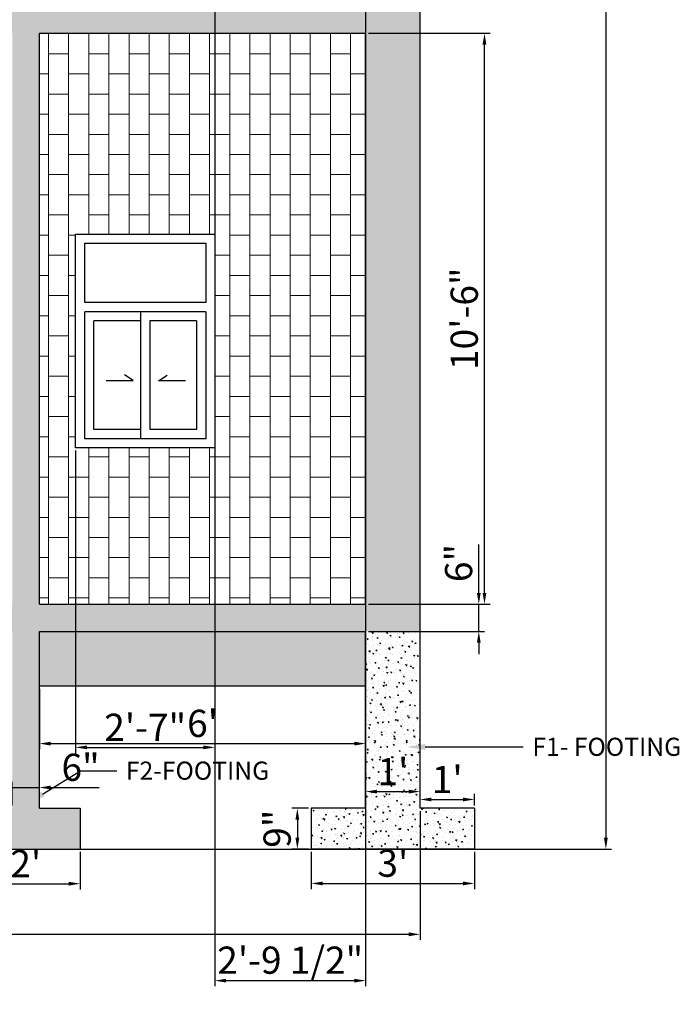
# Model space of a CAD drawing. Units: millimetres. Extents: x 20768 to 23556, y 50760 to 52704.
# Tile 4 of 36: x 21124 to 21270, y 51066 to 51283. Entities that reach past the tile are written whole.
import ezdxf
from ezdxf import colors
from ezdxf.entities.mleader import LeaderData, LeaderLine
from ezdxf.math import Vec2, Vec3

# ---------------------------------------------------------------- set-up
doc = ezdxf.new("R2010")
doc.units = ezdxf.units.MM
for name, color, linetype, lineweight in [('A-ANNO-DIMS', 2, 'Continuous', 18), ('A-ANNO-TEXT', 7, 'Continuous', 18), ('A-ELEV', 7, 'Continuous', 25), ('A-ELEV-PATT', 8, 'Continuous', 13), ('S-ANNO-DIMS', 2, 'Continuous', 18)]:
    doc.layers.add(name, color=color, linetype=linetype, lineweight=lineweight)
doc.styles.get("Standard").update_dxf_attribs({"font": 'arial.ttf'})
doc.dimstyles.new('ISO-25', dxfattribs={"dimtxt": 6, "dimasz": 2.5, "dimexe": 1.25, "dimexo": 0.625, "dimtad": 1, "dimdec": 0, "dimlunit": 3, "dimtxsty": 'Standard', "dimcen": 2.5, "dimadec": 0, "dimazin": 0, "dimtfac": 1, "dimtdec": 0, "dimtmove": 0, "dimatfit": 3, "dimfxl": 1, "dimarcsym": 0})
pattern_1 = [(140, (105.777, 340.6355), (0.23908628, 2.732770035), [0.28575, -3.14325]), (85, (105.777, 340.6355), (-2.86585268, -0.52865132), [0.2286, -2.51460876]), (190.4514447, (105.797, 340.8633), (-2.62676628, 2.20411871), [0.24285013, -2.67135367]), (136.1842, (105.015, 340.6355), (0.63063492, 4.06618561), [0.428625, -4.714875]), (186.635558, (105.0677, 340.9744), (-3.71139187, 3.561062), [0.36427535, -4.00703412]), (81.184151, (105.015, 340.6355), (-3.71139187, 3.561062), [0.3428995, -3.77189598]), (111, (105.2056, 341.0165), (1.53397797, 2.27421587), [0.28575, -3.14325]), (56, (105.2056, 341.0165), (-2.76281949, 0.92703043), [0.2286, -2.5146]), (161.451445, (105.3334, 341.206), (-1.22884153, 3.20124629), [0.24285013, -2.67134906]), (127.5, (105.7771, 340.6355), (-1.268325583, 0.046329049), [0, -2.48412, 0, -2.5527, 0, -2.524125]), (97.5, (105.7771, 340.6355), (-1.502708622, 1.002294938), [0, -1.45542, 0, -2.42697, 0, -0.962025]), (57.5, (105.7771, 339.7859), (0.08593116, 2.033858928), [0, -0.9525, 0, -2.9718, 0, -3.94335]), (47.5, (105.7771, 339.4049), (-0.381397365, 2.22193772), [0, -1.23825, 0, -1.97358, 0, -2.80035])]

# ---------------------------------------------------------------- blocks, each defined once
blk = doc.blocks.new('*D134')
at = {"layer": 'A-ANNO-DIMS', "color": 0, "lineweight": -2, "transparency": 16777216}
for p, q in [((21128.63, 51135.87), (21128.63, 51122.52)), ((21200.63, 51135.87), (21200.63, 51122.52)), ((21131.13, 51123.77), (21198.13, 51123.77))]:
    blk.add_line(p, q, dxfattribs=at)
at = {"layer": 'A-ANNO-DIMS', "color": 0, "transparency": 16777216}
for points in [[(21131.13, 51124.18), (21131.13, 51123.35), (21128.63, 51123.77)], [(21198.13, 51124.18), (21198.13, 51123.35), (21200.63, 51123.77)]]:
    blk.add_solid(points, dxfattribs=at)
at = {"layer": 'Defpoints', "color": 0, "transparency": 16777216}
for p in [(21128.63, 51136.5), (21200.63, 51136.5), (21200.63, 51123.77)]:
    blk.add_point(p, dxfattribs=at)
at = {"layer": 'A-ANNO-DIMS', "color": 0, "transparency": 16777216, "insert": (21164.63, 51127.45), "char_height": 6, "attachment_point": 5}
blk.add_mtext("6'", dxfattribs=at)
blk = doc.blocks.new('*D135')
at = {"layer": 'A-ANNO-DIMS', "color": 0, "lineweight": -2, "transparency": 16777216}
for p, q in [((21122.63, 51110.12), (21122.63, 51115.33)), ((21128.63, 51110.12), (21128.63, 51115.33)), ((21120.13, 51114.08), (21117.63, 51114.08)), ((21122.63, 51114.08), (21128.63, 51114.08)), ((21131.13, 51114.08), (21141.81, 51114.08))]:
    blk.add_line(p, q, dxfattribs=at)
at = {"layer": 'A-ANNO-DIMS', "color": 0, "transparency": 16777216}
for points in [[(21120.13, 51114.5), (21120.13, 51113.66), (21122.63, 51114.08)], [(21131.13, 51114.5), (21131.13, 51113.66), (21128.63, 51114.08)]]:
    blk.add_solid(points, dxfattribs=at)
at = {"layer": 'Defpoints', "color": 0, "transparency": 16777216}
for p in [(21128.63, 51114.08), (21122.63, 51109.5), (21128.63, 51109.5)]:
    blk.add_point(p, dxfattribs=at)
at = {"layer": 'A-ANNO-DIMS', "color": 0, "transparency": 16777216, "insert": (21137.72, 51117.77), "char_height": 6, "attachment_point": 5}
blk.add_mtext('6"', dxfattribs=at)
blk = doc.blocks.new('*D136')
at = {"layer": 'A-ANNO-DIMS', "color": 0, "lineweight": -2, "transparency": 16777216}
for p, q in [((21113.63, 51099.87), (21113.63, 51091.63)), ((21137.63, 51099.87), (21137.63, 51091.63)), ((21116.13, 51092.88), (21135.13, 51092.88))]:
    blk.add_line(p, q, dxfattribs=at)
at = {"layer": 'A-ANNO-DIMS', "color": 0, "transparency": 16777216}
for points in [[(21116.13, 51093.29), (21116.13, 51092.46), (21113.63, 51092.88)], [(21135.13, 51093.29), (21135.13, 51092.46), (21137.63, 51092.88)]]:
    blk.add_solid(points, dxfattribs=at)
at = {"layer": 'Defpoints', "color": 0, "transparency": 16777216}
for p in [(21113.63, 51100.5), (21137.63, 51100.5), (21137.63, 51092.88)]:
    blk.add_point(p, dxfattribs=at)
at = {"layer": 'A-ANNO-DIMS', "color": 0, "transparency": 16777216, "insert": (21125.63, 51096.52), "char_height": 6, "attachment_point": 5}
blk.add_mtext("2'", dxfattribs=at)
blk = doc.blocks.new('*D138')
at = {"layer": 'A-ANNO-DIMS', "color": 0, "lineweight": -2, "transparency": 16777216}
for p, q in [((21188.01, 51109.5), (21184.31, 51109.5)), ((21185.56, 51107), (21185.56, 51103)), ((21188.01, 51100.5), (21184.31, 51100.5))]:
    blk.add_line(p, q, dxfattribs=at)
at = {"layer": 'A-ANNO-DIMS', "color": 0, "transparency": 16777216}
for points in [[(21185.14, 51107), (21185.97, 51107), (21185.56, 51109.5)], [(21185.14, 51103), (21185.97, 51103), (21185.56, 51100.5)]]:
    blk.add_solid(points, dxfattribs=at)
at = {"layer": 'Defpoints', "color": 0, "transparency": 16777216}
for p in [(21188.63, 51109.5), (21185.56, 51100.5), (21188.63, 51100.5)]:
    blk.add_point(p, dxfattribs=at)
at = {"layer": 'A-ANNO-DIMS', "color": 0, "transparency": 16777216, "insert": (21181.87, 51105), "char_height": 6, "attachment_point": 5, "rotation": 90}
blk.add_mtext('9"', dxfattribs=at)
blk = doc.blocks.new('*D139')
at = {"layer": 'A-ANNO-DIMS', "color": 0, "lineweight": -2, "transparency": 16777216}
for p, q in [((21200.63, 51110.12), (21200.63, 51114.43)), ((21212.63, 51110.12), (21212.63, 51114.43)), ((21203.13, 51113.18), (21210.13, 51113.18))]:
    blk.add_line(p, q, dxfattribs=at)
at = {"layer": 'A-ANNO-DIMS', "color": 0, "transparency": 16777216}
for points in [[(21203.13, 51113.6), (21203.13, 51112.77), (21200.63, 51113.18)], [(21210.13, 51113.6), (21210.13, 51112.77), (21212.63, 51113.18)]]:
    blk.add_solid(points, dxfattribs=at)
at = {"layer": 'Defpoints', "color": 0, "transparency": 16777216}
for p in [(21212.63, 51113.18), (21200.63, 51109.5), (21212.63, 51109.5)]:
    blk.add_point(p, dxfattribs=at)
at = {"layer": 'A-ANNO-DIMS', "color": 0, "transparency": 16777216, "insert": (21206.63, 51116.82), "char_height": 6, "attachment_point": 5}
blk.add_mtext("1'", dxfattribs=at)
blk = doc.blocks.new('*D140')
at = {"layer": 'A-ANNO-DIMS', "color": 0, "lineweight": -2, "transparency": 16777216}
for p, q in [((21212.63, 51110.12), (21212.63, 51112.7)), ((21224.63, 51110.12), (21224.63, 51112.7)), ((21215.13, 51111.45), (21222.13, 51111.45))]:
    blk.add_line(p, q, dxfattribs=at)
at = {"layer": 'A-ANNO-DIMS', "color": 0, "transparency": 16777216}
for points in [[(21215.13, 51111.86), (21215.13, 51111.03), (21212.63, 51111.45)], [(21222.13, 51111.86), (21222.13, 51111.03), (21224.63, 51111.45)]]:
    blk.add_solid(points, dxfattribs=at)
at = {"layer": 'Defpoints', "color": 0, "transparency": 16777216}
for p in [(21224.63, 51111.45), (21212.63, 51109.5), (21224.63, 51109.5)]:
    blk.add_point(p, dxfattribs=at)
at = {"layer": 'A-ANNO-DIMS', "color": 0, "transparency": 16777216, "insert": (21218.63, 51115.08), "char_height": 6, "attachment_point": 5}
blk.add_mtext("1'", dxfattribs=at)
blk = doc.blocks.new('*D141')
at = {"layer": 'A-ANNO-DIMS', "color": 0, "lineweight": -2, "transparency": 16777216}
for p, q in [((21188.63, 51099.87), (21188.63, 51091.68)), ((21224.63, 51099.87), (21224.63, 51091.68)), ((21191.13, 51092.93), (21222.13, 51092.93))]:
    blk.add_line(p, q, dxfattribs=at)
at = {"layer": 'A-ANNO-DIMS', "color": 0, "transparency": 16777216}
for points in [[(21191.13, 51093.35), (21191.13, 51092.51), (21188.63, 51092.93)], [(21222.13, 51093.35), (21222.13, 51092.51), (21224.63, 51092.93)]]:
    blk.add_solid(points, dxfattribs=at)
at = {"layer": 'Defpoints', "color": 0, "transparency": 16777216}
for p in [(21188.63, 51100.5), (21224.63, 51100.5), (21224.63, 51092.93)]:
    blk.add_point(p, dxfattribs=at)
at = {"layer": 'A-ANNO-DIMS', "color": 0, "transparency": 16777216, "insert": (21206.63, 51096.62), "char_height": 6, "attachment_point": 5}
blk.add_mtext("3'", dxfattribs=at)
blk = doc.blocks.new('*D113')
at = {"layer": 'A-ANNO-DIMS', "color": 0, "lineweight": -2, "transparency": 16777216}
for p, q in [((21225.6, 51157), (21225.6, 51167.68)), ((21201.26, 51154.5), (21226.85, 51154.5)), ((21225.6, 51148.5), (21225.6, 51154.5)), ((21201.26, 51148.5), (21226.85, 51148.5)), ((21225.6, 51146), (21225.6, 51143.5))]:
    blk.add_line(p, q, dxfattribs=at)
at = {"layer": 'A-ANNO-DIMS', "color": 0, "transparency": 16777216}
for points in [[(21225.18, 51157), (21226.01, 51157), (21225.6, 51154.5)], [(21225.18, 51146), (21226.01, 51146), (21225.6, 51148.5)]]:
    blk.add_solid(points, dxfattribs=at)
at = {"layer": 'Defpoints', "color": 0, "transparency": 16777216}
for p in [(21200.63, 51154.5), (21225.6, 51154.5), (21200.63, 51148.5)]:
    blk.add_point(p, dxfattribs=at)
at = {"layer": 'A-ANNO-DIMS', "color": 0, "transparency": 16777216, "insert": (21221.91, 51163.59), "char_height": 6, "attachment_point": 5, "rotation": 90}
blk.add_mtext('6"', dxfattribs=at)
blk = doc.blocks.new('*D114')
at = {"layer": 'A-ANNO-DIMS', "color": 0, "lineweight": -2, "transparency": 16777216}
for p, q in [((21201.26, 51280.4), (21228.1, 51280.4)), ((21226.85, 51157), (21226.85, 51277.9)), ((21201.26, 51154.5), (21228.1, 51154.5))]:
    blk.add_line(p, q, dxfattribs=at)
at = {"layer": 'A-ANNO-DIMS', "color": 0, "transparency": 16777216}
for points in [[(21226.43, 51277.9), (21227.26, 51277.9), (21226.85, 51280.4)], [(21226.43, 51157), (21227.26, 51157), (21226.85, 51154.5)]]:
    blk.add_solid(points, dxfattribs=at)
at = {"layer": 'Defpoints', "color": 0, "transparency": 16777216}
for p in [(21200.63, 51280.4), (21226.85, 51280.4), (21200.63, 51154.5)]:
    blk.add_point(p, dxfattribs=at)
at = {"layer": 'A-ANNO-DIMS', "color": 0, "transparency": 16777216, "insert": (21223.16, 51217.45), "char_height": 6, "attachment_point": 5, "rotation": 90}
blk.add_mtext('10\'-6"', dxfattribs=at)
blk = doc.blocks.new('*D123')
at = {"layer": 'A-ANNO-DIMS', "color": 0, "lineweight": -2, "transparency": 16777216}
for p, q in [((21136.63, 51188.37), (21136.63, 51121.69)), ((21167.33, 51188.37), (21167.33, 51121.69)), ((21139.13, 51122.94), (21164.83, 51122.94))]:
    blk.add_line(p, q, dxfattribs=at)
at = {"layer": 'A-ANNO-DIMS', "color": 0, "transparency": 16777216}
for points in [[(21139.13, 51123.35), (21139.13, 51122.52), (21136.63, 51122.94)], [(21164.83, 51123.35), (21164.83, 51122.52), (21167.33, 51122.94)]]:
    blk.add_solid(points, dxfattribs=at)
at = {"layer": 'Defpoints', "color": 0, "transparency": 16777216}
for p in [(21136.63, 51189), (21167.33, 51189), (21167.33, 51122.94)]:
    blk.add_point(p, dxfattribs=at)
at = {"layer": 'A-ANNO-DIMS', "color": 0, "transparency": 16777216, "insert": (21151.98, 51126.58), "char_height": 6, "attachment_point": 5}
blk.add_mtext('2\'-7"', dxfattribs=at)
blk = doc.blocks.new('*D111')
at = {"layer": 'A-ANNO-DIMS', "color": 0, "lineweight": -2, "transparency": 16777216}
for p, q in [((20972.63, 51108.87), (20972.63, 51080.46)), ((21212.63, 51108.87), (21212.63, 51080.46)), ((20975.13, 51081.71), (21210.13, 51081.71))]:
    blk.add_line(p, q, dxfattribs=at)
at = {"layer": 'A-ANNO-DIMS', "color": 0, "transparency": 16777216}
for points in [[(20975.13, 51082.13), (20975.13, 51081.29), (20972.63, 51081.71)], [(21210.13, 51082.13), (21210.13, 51081.29), (21212.63, 51081.71)]]:
    blk.add_solid(points, dxfattribs=at)
at = {"layer": 'Defpoints', "color": 0, "transparency": 16777216}
for p in [(20972.63, 51109.5), (21212.63, 51109.5), (21212.63, 51081.71)]:
    blk.add_point(p, dxfattribs=at)
at = {"layer": 'A-ANNO-DIMS', "color": 0, "transparency": 16777216, "insert": (21092.63, 51085.4), "char_height": 6, "attachment_point": 5}
blk.add_mtext("20'", dxfattribs=at)
blk = doc.blocks.new('*D229')
at = {"layer": 'Defpoints', "color": 0, "transparency": 16777216}
for p in [(20963.6, 51532.3), (20960.63, 51100.5), (21253.63, 51100.5)]:
    blk.add_point(p, dxfattribs=at)
at = {"layer": 'S-ANNO-DIMS', "color": 0, "lineweight": -2, "transparency": 16777216}
for p, q in [((20964.22, 51532.3), (21254.88, 51532.3)), ((21253.63, 51529.8), (21253.63, 51103)), ((20961.26, 51100.5), (21254.88, 51100.5))]:
    blk.add_line(p, q, dxfattribs=at)
at = {"layer": 'S-ANNO-DIMS', "color": 0, "transparency": 16777216}
for points in [[(21253.22, 51529.8), (21254.05, 51529.8), (21253.63, 51532.3)], [(21253.22, 51103), (21254.05, 51103), (21253.63, 51100.5)]]:
    blk.add_solid(points, dxfattribs=at)
at = {"layer": 'S-ANNO-DIMS', "color": 0, "transparency": 16777216, "insert": (21249.94, 51316.4), "char_height": 6, "attachment_point": 5, "rotation": 90}
blk.add_mtext('36\'-0"', dxfattribs=at)
blk = doc.blocks.new('*D231')
at = {"layer": 'Defpoints', "color": 0, "transparency": 16777216}
for p in [(21167.33, 51320.9), (21200.63, 51286.4), (21200.63, 51071.5)]:
    blk.add_point(p, dxfattribs=at)
at = {"layer": 'S-ANNO-DIMS', "color": 0, "lineweight": -2, "transparency": 16777216}
for p, q in [((21167.33, 51320.27), (21167.33, 51070.25)), ((21200.63, 51285.77), (21200.63, 51070.25)), ((21169.83, 51071.5), (21198.13, 51071.5))]:
    blk.add_line(p, q, dxfattribs=at)
at = {"layer": 'S-ANNO-DIMS', "color": 0, "transparency": 16777216}
for points in [[(21169.83, 51071.91), (21169.83, 51071.08), (21167.33, 51071.5)], [(21198.13, 51071.91), (21198.13, 51071.08), (21200.63, 51071.5)]]:
    blk.add_solid(points, dxfattribs=at)
at = {"layer": 'S-ANNO-DIMS', "color": 0, "transparency": 16777216, "insert": (21183.98, 51075.23), "char_height": 6, "attachment_point": 5}
blk.add_mtext('2\'-9 1/2"', dxfattribs=at)

msp = doc.modelspace()

# ---------------------------------------------------------------- hatches: boundary and pattern name
at = {"layer": 'A-ELEV-PATT'}
h = msp.add_hatch(dxfattribs=at)
h.set_pattern_fill('AR-CONC', color=256, scale=0.015, angle=90)
h.set_pattern_definition(pattern_1)
h.paths.add_polyline_path([(21212.63, 51490.3), (21200.63, 51490.3), (21200.63, 51418.3), (21128.63, 51418.3), (21128.63, 51490.3), (21122.63, 51490.3), (21122.63, 51418.3), (20972.63, 51418.3), (20972.63, 51109.5), (20960.63, 51109.5), (20960.63, 51100.5), (20996.63, 51100.5), (20996.63, 51109.5), (20984.63, 51109.5), (20984.63, 51148.5), (21122.63, 51148.5), (21122.63, 51109.5), (21113.63, 51109.5), (21113.63, 51100.5), (21137.63, 51100.5), (21137.63, 51109.5), (21128.63, 51109.5), (21128.63, 51148.5), (21212.63, 51148.5)])
h.paths.add_polyline_path([(21122.63, 51280.4), (21122.63, 51154.5), (20984.63, 51154.5), (20984.63, 51280.4)], flags=16)
h.paths.add_polyline_path([(21122.63, 51286.4), (20984.63, 51286.4), (20984.63, 51412.3), (21122.63, 51412.3)], flags=16)
h.paths.add_polyline_path([(21128.63, 51280.4), (21200.63, 51280.4), (21200.63, 51154.5), (21128.63, 51154.5)], flags=16)
h.paths.add_polyline_path([(21128.63, 51286.4), (21128.63, 51412.3), (21200.63, 51412.3), (21200.63, 51286.4)], flags=16)
h.paths.add_polyline_path([(21062.79, 51358.4), (21062.79, 51361.4), (21118.63, 51361.4), (21118.63, 51358.4)], flags=0)
h.paths.add_polyline_path([(21111.63, 51320.9), (21090.63, 51286.4), (21069.63, 51320.9), (21069.63, 51355.4), (21111.63, 51355.4)], flags=0)
h.paths.add_polyline_path([(21069.63, 51320.9), (21090.63, 51355.4), (21111.63, 51320.9)], flags=0)
h.paths.add_polyline_path([(21136.63, 51320.9), (21136.63, 51368), (21167.33, 51368), (21167.33, 51320.9)], flags=0)
h.paths.add_polyline_path([(21138.63, 51322.9), (21138.63, 51350.9), (21165.33, 51350.9), (21165.33, 51322.9)], flags=0)
h.paths.add_polyline_path([(21140.63, 51324.9), (21140.63, 51348.9), (21150.98, 51348.9), (21150.98, 51324.9)], flags=0)
h.paths.add_polyline_path([(21136.63, 51236.1), (21167.33, 51236.1), (21167.33, 51189), (21136.63, 51189)], flags=0)
h.paths.add_polyline_path([(21152.98, 51324.9), (21152.98, 51348.9), (21163.33, 51348.9), (21163.33, 51324.9)], flags=0)
h.paths.add_polyline_path([(21094.84, 51323.58), (21094.21, 51323.58, -0.960515), (21092.46, 51323.65, -0.414214), (21093.33, 51324.52), (21093.33, 51325.09, -0.357901), (21093.11, 51325.35, -1), (21093.66, 51325.35, -0.34824), (21093.45, 51325.09), (21093.45, 51324.51, -0.376216), (21094.21, 51323.65), (21094.84, 51323.65)], flags=0)
h.paths.add_polyline_path([(21138.63, 51234.1), (21165.33, 51234.1), (21165.33, 51221), (21138.63, 51221)], flags=0)
h.paths.add_polyline_path([(21118.63, 51229.5), (21118.63, 51226.5), (21062.79, 51226.5), (21062.79, 51229.5)], flags=0)
h.paths.add_polyline_path([(21087.06, 51323.58), (21086.42, 51323.58), (21086.42, 51323.65), (21087.06, 51323.65, -0.376216), (21087.82, 51324.51), (21087.82, 51325.09, -0.34824), (21087.61, 51325.35, -1), (21088.15, 51325.35, -0.357901), (21087.94, 51325.09), (21087.94, 51324.52, -0.414214), (21088.81, 51323.65, -0.960515)], flags=0)
h.paths.add_polyline_path([(21111.63, 51223.5), (21111.63, 51189), (21090.63, 51154.5), (21069.63, 51189), (21069.63, 51223.5)], flags=0)
h.paths.add_polyline_path([(21138.63, 51219), (21165.33, 51219), (21165.33, 51191), (21138.63, 51191)], flags=0)
h.paths.add_polyline_path([(21140.63, 51217), (21150.98, 51217), (21150.98, 51193), (21140.63, 51193)], flags=0)
h.paths.add_polyline_path([(21056.63, 51166.5), (21020.63, 51166.5), (21020.63, 51214.5), (21056.63, 51214.5)], flags=0)
h.paths.add_polyline_path([(21056.63, 51298.4), (21020.63, 51298.4), (21020.63, 51346.4), (21056.63, 51346.4)], flags=0)
h.paths.add_polyline_path([(21090.63, 51223.5), (21111.63, 51189), (21069.63, 51189)], flags=0)
h.paths.add_polyline_path([(21138.63, 51352.9), (21138.63, 51366), (21165.33, 51366), (21165.33, 51352.9)], flags=0)
h.paths.add_polyline_path([(21152.98, 51217), (21163.33, 51217), (21163.33, 51193), (21152.98, 51193)], flags=0)
h.paths.add_polyline_path([(21093.66, 51193.45, -0.34824), (21093.45, 51193.19), (21093.45, 51192.61, -0.376216), (21094.21, 51191.75), (21094.84, 51191.75), (21094.84, 51191.68), (21094.21, 51191.68, -0.960515), (21092.46, 51191.75, -0.414214), (21093.33, 51192.62), (21093.33, 51193.19, -0.357901), (21093.11, 51193.45, -1)], flags=0)
h.paths.add_polyline_path([(21088.15, 51193.45, -0.357901), (21087.94, 51193.19), (21087.94, 51192.62, -0.414214), (21088.81, 51191.75, -0.960515), (21087.06, 51191.68), (21086.42, 51191.68), (21086.42, 51191.75), (21087.06, 51191.75, -0.376216), (21087.82, 51192.61), (21087.82, 51193.19, -0.34824), (21087.61, 51193.45, -1)], flags=0)
h = msp.add_hatch(dxfattribs=at)
h.set_pattern_fill('BRICK', color=256, scale=0.7, angle=90)
h.set_pattern_definition([(90, (105.777, 340.6355), (-4.445, 3e-16), []), (180, (105.777, 340.6355), (-1e-15, -8.89), [4.445, -4.445]), (180, (105.777, 345.0805), (-1e-15, -8.89), [-4.445, 4.445])])
h.paths.add_polyline_path([(21200.63, 51280.4), (21128.63, 51280.4), (21128.63, 51154.5), (21200.63, 51154.5)])
h.paths.add_polyline_path([(21167.33, 51236.1), (21167.33, 51189), (21136.63, 51189), (21136.63, 51236.1)], flags=16)
h.paths.add_polyline_path([(21165.33, 51234.1), (21165.33, 51221), (21138.63, 51221), (21138.63, 51234.1)], flags=0)
h.paths.add_polyline_path([(21165.33, 51219), (21165.33, 51191), (21138.63, 51191), (21138.63, 51219)], flags=0)
h.paths.add_polyline_path([(21163.33, 51217), (21163.33, 51193), (21152.98, 51193), (21152.98, 51217)], flags=0)
h.paths.add_polyline_path([(21150.98, 51193), (21140.63, 51193), (21140.63, 51217), (21150.98, 51217)], flags=0)
h = msp.add_hatch(dxfattribs=at)
h.set_pattern_fill('AR-CONC', color=256, scale=0.015, angle=90)
h.set_pattern_definition(pattern_1)
h.paths.add_polyline_path([(21200.63, 51148.5), (21128.63, 51148.5), (21128.63, 51136.5), (21200.63, 51136.5)])
h = msp.add_hatch(dxfattribs=at)
h.set_pattern_fill('AR-CONC', color=256, scale=0.015, angle=90)
h.set_pattern_definition(pattern_1)
h.paths.add_polyline_path([(21212.63, 51148.5), (21200.63, 51148.5), (21200.63, 51109.5), (21188.63, 51109.5), (21188.63, 51100.5), (21224.63, 51100.5), (21224.63, 51109.5), (21212.63, 51109.5)])

# ---------------------------------------------------------------- linework, layer by layer
at = {"layer": 'A-ELEV'}
for p, q in [((21212.63, 51109.5), (21212.63, 51490.3)), ((21128.63, 51154.5), (21128.63, 51280.4)), ((21128.63, 51280.4), (21200.63, 51280.4)), ((21200.63, 51154.5), (21200.63, 51280.4)), ((21136.63, 51236.1), (21167.33, 51236.1)), ((21136.63, 51189), (21136.63, 51236.1)), ((21167.33, 51236.1), (21167.33, 51189)), ((21165.33, 51219), (21138.63, 51219)), ((21138.63, 51191), (21138.63, 51219)), ((21150.98, 51219), (21150.98, 51191)), ((21165.33, 51219), (21165.33, 51191)), ((21150.98, 51217), (21140.63, 51217)), ((21140.63, 51193), (21140.63, 51217)), ((21163.33, 51217), (21152.98, 51217)), ((21152.98, 51217), (21152.98, 51193)), ((21163.33, 51217), (21163.33, 51193)), ((21143.34, 51203.85), (21149.32, 51203.85)), ((21149.32, 51203.85), (21147.43, 51205.06)), ((21154.92, 51203.78), (21156.81, 51204.99)), ((21160.9, 51203.78), (21154.92, 51203.78)), ((21150.98, 51193), (21140.63, 51193)), ((21163.33, 51193), (21152.98, 51193)), ((21165.33, 51191), (21138.63, 51191)), ((21167.33, 51189), (21136.63, 51189)), ((21128.63, 51154.5), (21200.63, 51154.5)), ((21128.63, 51109.5), (21128.63, 51148.5)), ((21128.63, 51148.5), (21200.63, 51148.5)), ((21200.63, 51109.5), (21200.63, 51148.5)), ((21128.63, 51136.5), (21200.63, 51136.5)), ((21128.63, 51109.5), (21137.63, 51109.5)), ((21137.63, 51109.5), (21137.63, 51100.5)), ((21200.63, 51109.5), (21188.63, 51109.5)), ((21188.63, 51109.5), (21188.63, 51100.5)), ((21224.63, 51109.5), (21212.63, 51109.5)), ((21224.63, 51109.5), (21224.63, 51100.5)), ((21113.63, 51100.5), (21137.63, 51100.5)), ((21224.63, 51100.5), (21188.63, 51100.5))]:
    msp.add_line(p, q, dxfattribs=at)
msp.add_lwpolyline([(21165.33, 51234.1), (21165.33, 51221), (21138.63, 51221), (21138.63, 51234.1)], close=True, dxfattribs=at)

# ---------------------------------------------------------------- dimensions: what is measured, and where the dimension line sits
at = {"layer": 'A-ANNO-DIMS'}
for base, p1, p2, picture, middle in [((21226.85, 51280.4), (21200.63, 51154.5), (21200.63, 51280.4), '*D114', (21223.16, 51217.45)), ((21225.6, 51154.5), (21200.63, 51148.5), (21200.63, 51154.5), '*D113', (21221.91, 51163.59)), ((21185.56, 51100.5), (21188.63, 51109.5), (21188.63, 51100.5), '*D138', (21181.87, 51105))]:
    dim = msp.add_linear_dim(base=base, p1=p1, p2=p2, angle=90, dimstyle='ISO-25', override={"dimclrd": 0, "dimclre": 0, "dimclrt": 0}, dxfattribs=at)
    dim.commit()
    dim.dimension.update_dxf_attribs({"geometry": picture, "text_midpoint": middle})
for base, p1, p2, picture, middle in [((21167.33, 51122.94), (21136.63, 51189), (21167.33, 51189), '*D123', (21151.98, 51126.58)), ((21200.63, 51123.77), (21128.63, 51136.5), (21200.63, 51136.5), '*D134', (21164.63, 51127.45)), ((21128.63, 51114.08), (21122.63, 51109.5), (21128.63, 51109.5), '*D135', (21137.72, 51117.77)), ((21212.63, 51113.18), (21200.63, 51109.5), (21212.63, 51109.5), '*D139', (21206.63, 51116.82)), ((21224.63, 51111.45), (21212.63, 51109.5), (21224.63, 51109.5), '*D140', (21218.63, 51115.08)), ((21212.63, 51081.71), (20972.63, 51109.5), (21212.63, 51109.5), '*D111', (21092.63, 51085.4)), ((21137.63, 51092.88), (21113.63, 51100.5), (21137.63, 51100.5), '*D136', (21125.63, 51096.52)), ((21224.63, 51092.93), (21188.63, 51100.5), (21224.63, 51100.5), '*D141', (21206.63, 51096.62))]:
    dim = msp.add_linear_dim(base=base, p1=p1, p2=p2, dimstyle='ISO-25', override={"dimclrd": 0, "dimclre": 0, "dimclrt": 0}, dxfattribs=at)
    dim.commit()
    dim.dimension.update_dxf_attribs({"geometry": picture, "text_midpoint": middle})
at = {"layer": 'S-ANNO-DIMS'}
dim = msp.add_linear_dim(base=(21253.63, 51100.5), p1=(20963.6, 51532.3), p2=(20960.63, 51100.5), angle=90, dimstyle='ISO-25', override={"dimdec": 1, "dimlfac": 1, "dimrnd": 0, "dimzin": 1, "dimdsep": 46, "dimlunit": 4, "dimfrac": 2}, dxfattribs=at)
dim.commit()
dim.dimension.update_dxf_attribs({"geometry": '*D229', "text_midpoint": (21249.94, 51316.4)})
dim = msp.add_linear_dim(base=(21200.63, 51071.5), p1=(21167.33, 51320.9), p2=(21200.63, 51286.4), dimstyle='ISO-25', override={"dimdec": 1, "dimlfac": 1, "dimrnd": 0, "dimzin": 1, "dimdsep": 46, "dimlunit": 4, "dimfrac": 2}, dxfattribs=at)
dim.commit()
dim.dimension.update_dxf_attribs({"geometry": '*D231', "text_midpoint": (21183.98, 51075.23)})

# ---------------------------------------------------------------- leaders
at = {"layer": 'A-ANNO-TEXT'}
ml = msp.add_multileader_mtext('Standard', dxfattribs=at)
ml.set_content('F1- FOOTING', color=256)
ml.set_leader_properties()
ml.build(insert=Vec2(0, 0))
ctx = ml.context
ctx.base_point, ctx.plane_origin = Vec3(21235.41, 51123.02), Vec3(21209.79, 51123.02)
notes = []
notes.append((ctx, [(0, (1, 1, 0), (21227.41, 51123.02), (1, 0), 8, [(0, [(21209.79, 51123.02)], 0, [])])]))
ctx.mtext.insert, ctx.mtext.flow_direction = Vec3(21237.41, 51125.06), 5
ml = msp.add_multileader_mtext('Standard', dxfattribs=at)
ml.set_content('F2-FOOTING', color=256)
ml.set_leader_properties()
ml.build(insert=Vec2(0, 0))
ctx = ml.context
ctx.base_point, ctx.plane_origin = Vec3(21145.72, 51117.77), Vec3(21125.93, 51110.51)
notes.append((ctx, [(0, (1, 1, 0), (21137.72, 51117.77), (1, 0), 8, [(0, [(21125.93, 51110.51)], 0, [])])]))
ctx.mtext.insert, ctx.mtext.flow_direction = Vec3(21147.72, 51119.8), 5
for ctx, leaders in notes:
    for number, flags, end, landing, length, lines in leaders:
        leader = LeaderData()
        leader.index, (leader.has_last_leader_line, leader.has_dogleg_vector, leader.attachment_direction) = number, flags
        leader.last_leader_point, leader.dogleg_vector, leader.dogleg_length = Vec3(end), Vec3(landing), length
        for number, points, colour, breaks in lines:
            line = LeaderLine()
            line.index, line.vertices, line.color, line.breaks = number, Vec3.list(points), colors.encode_raw_color(colour), breaks
            leader.lines.append(line)
        ctx.leaders.append(leader)

doc.saveas('drawing.dxf')
